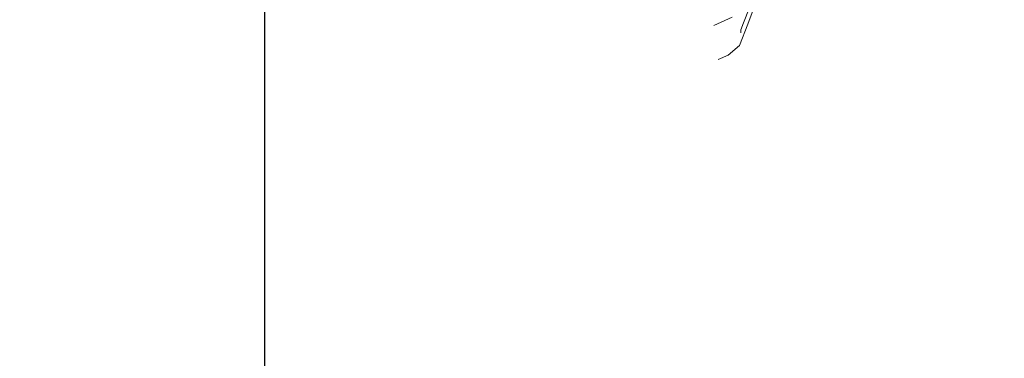
# Model space of a CAD drawing. Units: millimetres. Extents: x 595116 to 630915, y 909473 to 920225.
# Tile 54 of 134: x 629589 to 629609, y 919281 to 919288. Entities that reach past the tile are written whole.
import ezdxf

# ---------------------------------------------------------------- set-up
doc = ezdxf.new("R2010")
doc.units = ezdxf.units.MM
doc.layers.add('Dimension', color=3, linetype='Continuous', lineweight=18)
doc.layers.add('L-PLNT', color=85, linetype='Continuous', lineweight=13)
doc.styles.get("Standard").update_dxf_attribs({"font": 'arial.ttf'})
doc.dimstyles.new('ISO-25', dxfattribs={"dimtxt": 9, "dimasz": 6, "dimexe": 1.25, "dimexo": 0.625, "dimtad": 1, "dimlunit": 4, "dimtxsty": 'Standard', "dimcen": 2.5, "dimadec": 0, "dimazin": 0, "dimtfac": 1, "dimtmove": 0, "dimatfit": 3, "dimfxl": 1, "dimarcsym": 0})

# ---------------------------------------------------------------- blocks, each defined once
blk = doc.blocks.new('A$C4FB75ABC')
for p, q in [((3.2945, 0.3964), (3.2182, 0.1906)), ((3.2259, 0.2744), (3.1954, 0.1982)), ((3.1344, 0.2287), (3.0352, 0.1829)), ((3.2182, 0.1906), (3.1725, 0.0762)), ((3.1954, 0.1982), (3.1801, 0.1601)), ((3.1801, 0.1601), (3.1801, 0.1448)), ((3.1725, 0.0762), (3.1115, 0.0229)), ((3.1115, 0.0229), (3.0581, 0))]:
    blk.add_line(p, q)
blk = doc.blocks.new('*D210')
at = {"layer": 'Defpoints', "color": 0, "transparency": 16777216}
for p in [(629586.227, 919310.123), (629593.946, 919310.123), (629586.227, 919258.662)]:
    blk.add_point(p, dxfattribs=at)
at = {"layer": 'Dimension', "color": 0, "lineweight": -2, "transparency": 16777216}
for p, q in [((629593.946, 919310.123), (629593.946, 919449.69)), ((629586.852, 919310.123), (629595.196, 919310.123)), ((629593.946, 919264.662), (629593.946, 919304.123)), ((629586.852, 919258.662), (629595.196, 919258.662))]:
    blk.add_line(p, q, dxfattribs=at)
at = {"layer": 'Dimension', "color": 0, "transparency": 16777216}
for points in [[(629592.946, 919304.123), (629594.946, 919304.123), (629593.946, 919310.123)], [(629592.946, 919264.662), (629594.946, 919264.662), (629593.946, 919258.662)]]:
    blk.add_solid(points, dxfattribs=at)
at = {"layer": 'Dimension', "color": 0, "transparency": 16777216, "insert": (629588.662, 919382.907), "char_height": 9, "attachment_point": 5, "rotation": 90}
blk.add_mtext('CANOPY 4\'-3 1/2" TYP.', dxfattribs=at)
blk = doc.blocks.new('*D216')
at = {"layer": 'Defpoints', "color": 0, "transparency": 16777216}
for p in [(629743.541, 919411.928), (629505.041, 919411.828), (629743.541, 918832.378)]:
    blk.add_point(p, dxfattribs=at)
at = {"layer": 'Dimension', "color": 0, "lineweight": -2, "transparency": 16777216}
for p, q in [((629743.541, 919411.303), (629743.541, 918831.128)), ((629505.041, 919411.203), (629505.041, 918831.128)), ((629511.041, 918832.378), (629737.541, 918832.378))]:
    blk.add_line(p, q, dxfattribs=at)
at = {"layer": 'Dimension', "color": 0, "transparency": 16777216}
for points in [[(629511.041, 918833.378), (629511.041, 918831.378), (629505.041, 918832.378)], [(629737.541, 918833.378), (629737.541, 918831.378), (629743.541, 918832.378)]]:
    blk.add_solid(points, dxfattribs=at)
at = {"layer": 'Dimension', "color": 0, "transparency": 16777216, "insert": (629624.291, 918837.656), "char_height": 9, "attachment_point": 5}
blk.add_mtext('19\'-10 1/2"', dxfattribs=at)

msp = doc.modelspace()

# ---------------------------------------------------------------- block references
at = {"layer": 'L-PLNT', "xscale": 3.753413438031968, "yscale": 3.753413438031968, "zscale": 3.753413438031968}
msp.add_blockref('A$C4FB75ABC', (629591.653, 919287.212), dxfattribs=at)

# ---------------------------------------------------------------- dimensions: what is measured, and where the dimension line sits
at = {"layer": 'Dimension'}
dim = msp.add_linear_dim(base=(629593.946, 919310.123), p1=(629586.227, 919258.662), p2=(629586.227, 919310.123), angle=90, text='CANOPY <> TYP.', dimstyle='ISO-25', override={"dimdec": 1, "dimlfac": 1, "dimrnd": 0, "dimzin": 1, "dimdsep": 46, "dimlunit": 4, "dimfrac": 2}, dxfattribs=at)
dim.commit()
dim.dimension.update_dxf_attribs({"geometry": '*D210', "text_midpoint": (629588.662, 919382.907)})
dim = msp.add_linear_dim(base=(629743.541, 918832.378), p1=(629505.041, 919411.828), p2=(629743.541, 919411.928), dimstyle='ISO-25', override={"dimdec": 1, "dimlfac": 1, "dimrnd": 0, "dimzin": 1, "dimdsep": 46, "dimlunit": 4, "dimfrac": 2}, dxfattribs=at)
dim.commit()
dim.dimension.update_dxf_attribs({"geometry": '*D216', "text_midpoint": (629624.291, 918837.656)})

doc.saveas('drawing.dxf')
